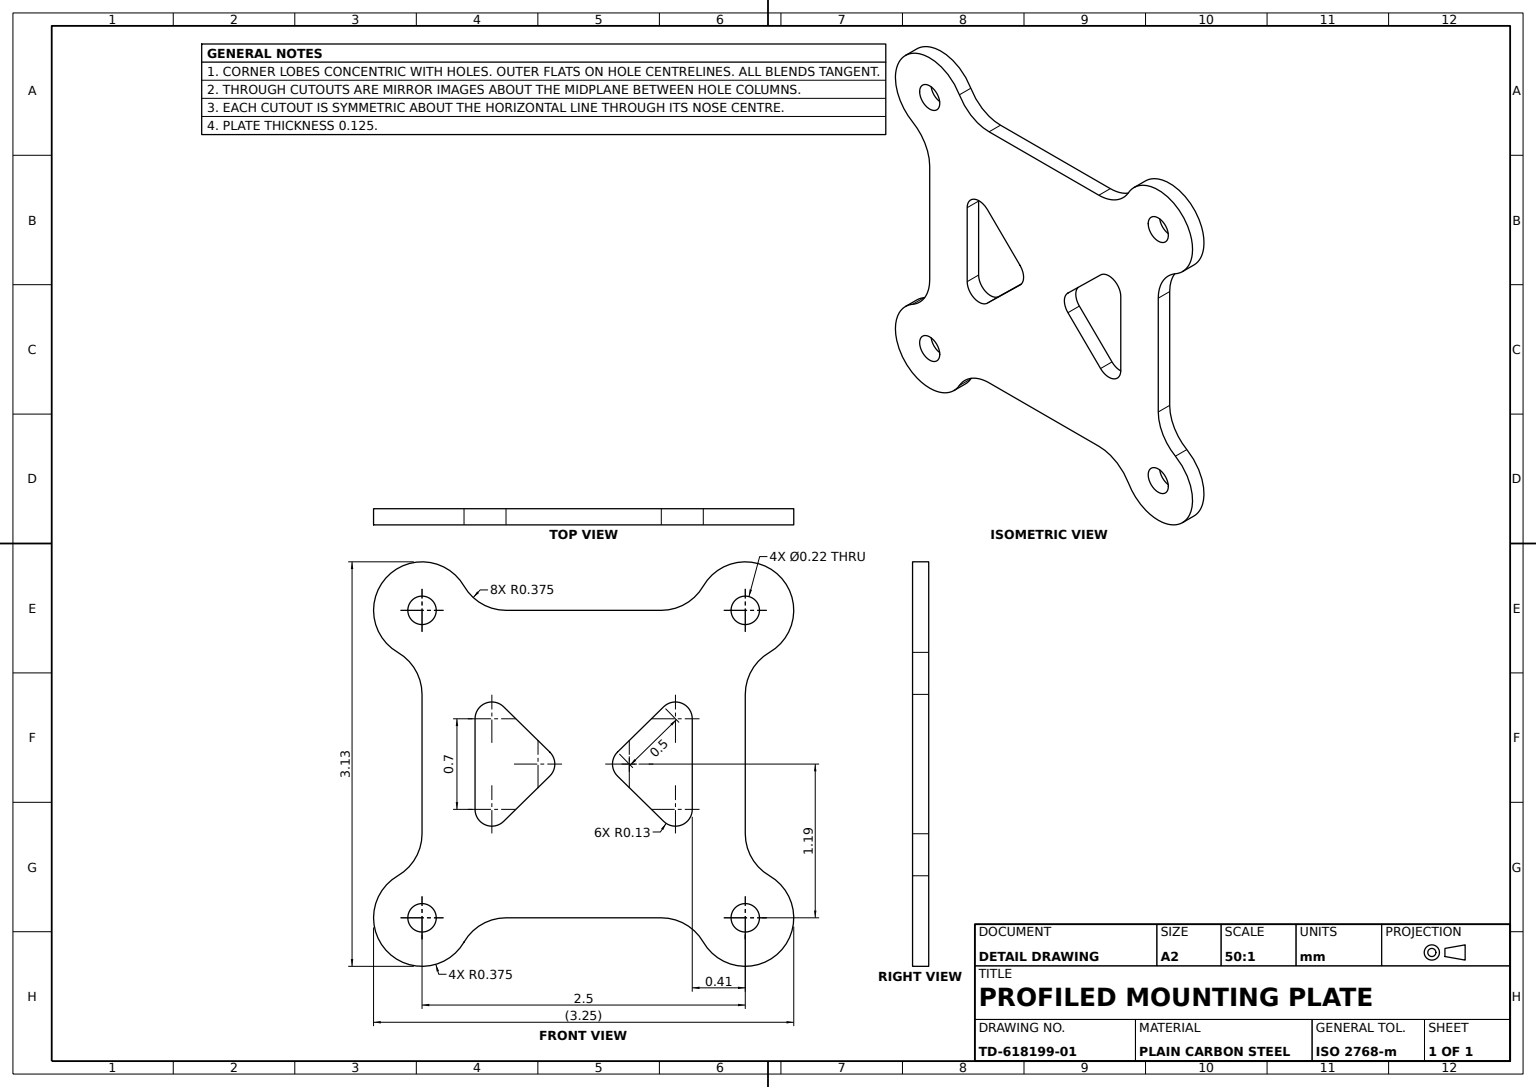
SolidWorks part; units mm, degrees
material "Plain Carbon Steel"
ref_plane "Front Plane" through (0, 0, 0) normal (0, 0, 1) x (1, 0, 0)
ref_plane "Top Plane" through (0, 0, 0) normal (0, 1, 0) x (1, 0, 0)
ref_plane "Right Plane" through (0, 0, 0) normal (1, 0, 0) x (0, 0, -1)
sketch "Bracket Plate Profile" plane through (0, 0, 0) normal (0, 0, 1) x (1, 0, 0)
  line L0 (0, 4.3513) -> (0, -4.6616) construction
  line L1 (-7.306, 0) -> (8.1466, 0) construction
  line L2 (-1.25, 0.5385) -> (-1.25, -0.5385)
  line L3 (1.25, 0.5385) -> (1.25, -0.5385)
  line L4 (-0.6005, -1.188) -> (0.6005, -1.188)
  line L5 (-0.6005, 1.188) -> (0.6005, 1.188)
  line L12 (-0.84, 0.35) -> (-0.84, -0.35)
  line L13 (-0.619, -0.4428) -> (-0.2619, -0.0928)
  line L14 (-0.2619, 0.0928) -> (-0.619, 0.4428)
  line L15 (0.619, -0.4428) -> (0.2619, -0.0928)
  line L16 (0.84, 0.35) -> (0.84, -0.35)
  line L17 (0.2619, 0.0928) -> (0.619, 0.4428)
  arc A0 (-0.9252, 1.3755) -> (-1.4375, 0.8632) centre (-1.25, 1.188) ccw
  circle A1 centre (-1.25, 1.188) radius 0.11
  arc A2 (1.4375, 0.8632) -> (0.9252, 1.3755) centre (1.25, 1.188) ccw
  circle A3 centre (1.25, 1.188) radius 0.11
  circle A4 centre (1.25, -1.188) radius 0.11
  arc A5 (1.4375, -0.8632) -> (0.9252, -1.3755) centre (1.25, -1.188) cw
  circle A6 centre (-1.25, -1.188) radius 0.11
  arc A7 (-0.9252, -1.3755) -> (-1.4375, -0.8632) centre (-1.25, -1.188) cw
  arc A8 (-1.25, 0.5385) -> (-1.4375, 0.8632) centre (-1.625, 0.5385) ccw
  arc A9 (1.25, 0.5385) -> (1.4375, 0.8632) centre (1.625, 0.5385) cw
  arc A10 (1.25, -0.5385) -> (1.4375, -0.8632) centre (1.625, -0.5385) ccw
  arc A11 (-1.25, -0.5385) -> (-1.4375, -0.8632) centre (-1.625, -0.5385) cw
  arc A12 (-0.9252, 1.3755) -> (-0.6005, 1.188) centre (-0.6005, 1.563) ccw
  arc A13 (0.9252, 1.3755) -> (0.6005, 1.188) centre (0.6005, 1.563) cw
  arc A14 (0.9252, -1.3755) -> (0.6005, -1.188) centre (0.6005, -1.563) ccw
  arc A15 (-0.9252, -1.3755) -> (-0.6005, -1.188) centre (-0.6005, -1.563) cw
  arc A22 (-0.84, -0.35) -> (-0.619, -0.4428) centre (-0.71, -0.35) ccw
  arc A23 (-0.619, 0.4428) -> (-0.84, 0.35) centre (-0.71, 0.35) ccw
  arc A24 (-0.2619, 0.0928) -> (-0.2619, -0.0928) centre (-0.3529, 0) cw
  arc A25 (0.84, -0.35) -> (0.619, -0.4428) centre (0.71, -0.35) cw
  arc A26 (0.619, 0.4428) -> (0.84, 0.35) centre (0.71, 0.35) cw
  arc A27 (0.2619, 0.0928) -> (0.2619, -0.0928) centre (0.3529, 0) ccw
  point P17 (-0.84, 0)
  point P47 (-0.1672, 0)
  dimension "D1" = 0.375
  dimension "D2" = 0.22
  dimension "D5" = 0.375
  dimension "D7" = 0.13
  dimension "D8" = 0.13
  dimension "D9" = 0.41
  dimension "D6" = 0.13
  dimension "D3" = 2.5
  dimension "D4" = 1.188
  dimension "D10" = 0.5
  dimension "D11" = 0.7
  dimension "D12" = 2.376
extrude "Bracket Plate" add sketch "Bracket Plate Profile" along normal blind 0.125 contours A24 L14 A23 L12 A22 L13 | L17 A27 L15 A25 L16 A26 | A3 | A1 | A6 | A4 | L5 A13 A2 A9 L3 A10 A5 A14 L4 A15 A7 A11 L2 A8 A0 A12
